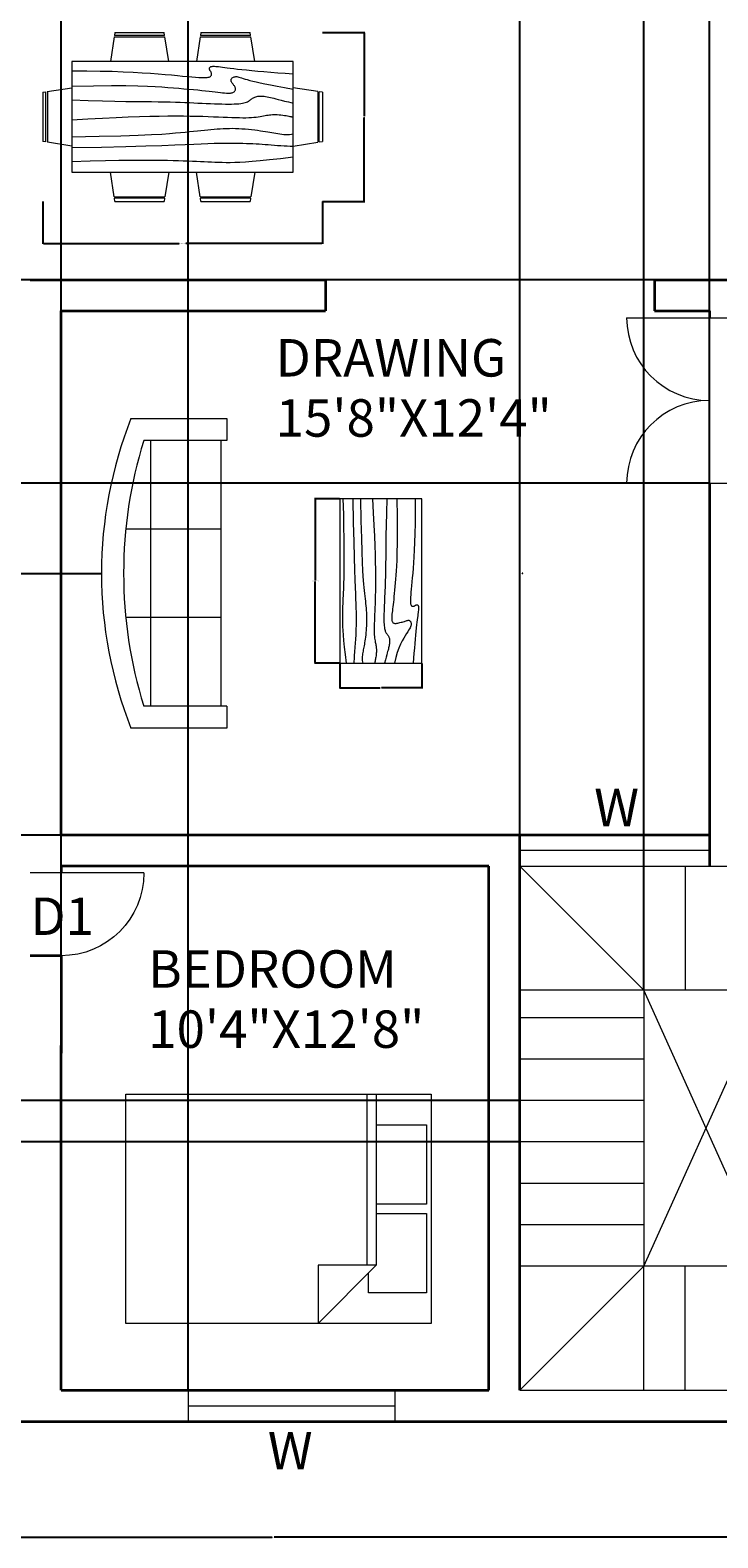
# Model space of a CAD drawing. Units: feet. Extents: x 1681 to 2398, y 1737 to 2411.
# Tile 2 of 4: x 1957 to 2156, y 1737 to 2174. Entities that reach past the tile are written whole.
import ezdxf

# ---------------------------------------------------------------- set-up
doc = ezdxf.new("R2010")
doc.units = ezdxf.units.FT
for name, color, linetype, lineweight in [('A-ANNO-DIMS', 2, 'Continuous', 18), ('A-ANNO-TEXT', 7, 'Continuous', 18), ('A-AREA-IDEN', 7, 'Continuous', 18), ('A-DOOR', 3, 'Continuous', 18), ('A-FLOR', 7, 'Continuous', 25), ('A-FLOR-STRS', 7, 'Continuous', 18), ('A-FURN', 8, 'Continuous', 13), ('A-GLAZ', 4, 'Continuous', 18), ('A-WALL', 7, 'Continuous', 35)]:
    doc.layers.add(name, color=color, linetype=linetype, lineweight=lineweight)
doc.styles.get("Standard").update_dxf_attribs({"font": 'arial.ttf'})
doc.dimstyles.get("Standard").update_dxf_attribs({"dimtxt": 0.18, "dimasz": 0.18, "dimexe": 0.18, "dimexo": 0.0625, "dimgap": 0.09, "dimtad": 0, "dimtih": 1, "dimtoh": 1, "dimdec": 4, "dimzin": 0, "dimdsep": 46, "dimtxsty": 'Standard', "dimcen": 0.09, "dimadec": 0, "dimazin": 0, "dimtfac": 1, "dimtdec": 4, "dimtofl": 0, "dimtmove": 0, "dimatfit": 3, "dimfxl": 1, "dimtolj": 1, "dimtzin": 0, "dimarcsym": 0})

# ---------------------------------------------------------------- blocks, each defined once
blk = doc.blocks.new('Dining Set - 36 x 72 in.')
for p, q in [((-22.2343, 26.00059), (-23.4847, 17.99762)), ((-22.2304, 26), (-5.7608, 26)), ((-22, 27.5), (-22.1562, 26.50042)), ((-5.8416, 26.5), (-22.1534, 26.5)), ((-22, 27.5), (-6, 27.5)), ((-5.8437, 26.49966), (-6, 27.5)), ((-4.5152, 17.99762), (-5.7655, 25.99926)), ((5.7657, 26.00059), (4.5153, 17.99762)), ((5.7696, 26), (22.2392, 26)), ((6, 27.5), (5.8438, 26.50042)), ((22.1584, 26.5), (5.8466, 26.5)), ((6, 27.5), (22, 27.5)), ((22.1563, 26.49966), (22, 27.5)), ((23.4848, 17.99762), (22.2345, 25.99926)), ((36, 18), (-36, 18)), ((-36, 18), (-36, -18)), ((36, -18), (36, 18)), ((-45.5, 8), (-44.5004, 8.15617)), ((-45.5, 8), (-45.5, -8)), ((-44.5, -8.15843), (-44.5, 8.15338)), ((-44.0006, 8.23428), (-35.9976, 9.48474)), ((-44, 8.23041), (-44, -8.23915)), ((44.0006, 8.23428), (35.9976, 9.48474)), ((44, 8.23041), (44, -8.23915)), ((44.5, -8.15843), (44.5, 8.15338)), ((45.5, 8), (44.5005, 8.15617)), ((45.5, 8), (45.5, -8)), ((-44.4997, -8.15631), (-45.5, -8)), ((-35.9976, -9.48476), (-43.9993, -8.2345)), ((35.9976, -9.48476), (43.9993, -8.2345)), ((44.4997, -8.15631), (45.5, -8)), ((-36, -18), (36, -18)), ((-22.2343, -26.0006), (-23.4847, -17.99762)), ((-4.5152, -17.99762), (-5.7655, -25.99928)), ((5.7657, -26.0006), (4.5153, -17.99762)), ((23.4848, -17.99762), (22.2345, -25.99928)), ((-22.2304, -26), (-5.7608, -26)), ((-22, -27.5), (-22.1562, -26.50044)), ((-5.8416, -26.5), (-22.1534, -26.5)), ((-22, -27.5), (-6, -27.5)), ((-5.8437, -26.49967), (-6, -27.5)), ((5.7696, -26), (22.2392, -26)), ((6, -27.5), (5.8438, -26.50044)), ((22.1584, -26.5), (5.8466, -26.5)), ((6, -27.5), (22, -27.5)), ((22.1563, -26.49967), (22, -27.5))]:
    blk.add_line(p, q)
for points in [[(-36, 15), (-31.1772, 14.97754), (-26.8079, 14.91406), (-22.8538, 14.81543), (-19.276, 14.6875), (-16.0362, 14.53613), (-13.0957, 14.36718), (-10.4159, 14.18652), (-7.9583, 14), (-5.6904, 13.81315), (-3.6035, 13.63021), (-1.6954, 13.45508), (0.0365, 13.29166), (1.5945, 13.14388), (2.9811, 13.01562), (4.1988, 12.9108), (5.25, 12.83333), (6.1393, 12.78613), (6.8802, 12.76823), (7.4883, 12.77767), (7.9792, 12.8125), (8.3685, 12.87077), (8.6719, 12.95052), (8.9049, 13.0498), (9.0833, 13.16666), (9.2205, 13.29899), (9.3216, 13.44401), (9.3895, 13.59879), (9.4271, 13.76041), (9.4373, 13.92594), (9.4232, 14.09245), (9.3875, 14.257), (9.3333, 14.41666), (9.2638, 14.56917), (9.1836, 14.71484), (9.0975, 14.85465), (9.0104, 14.98958), (8.9272, 15.1206), (8.8529, 15.2487), (8.7922, 15.37483), (8.75, 15.5), (8.7305, 15.62467), (8.7344, 15.74739), (8.7617, 15.86621), (8.8125, 15.97916), (8.8867, 16.08431), (8.9844, 16.17968), (9.1055, 16.26334), (9.25, 16.33333), (9.4189, 16.38802), (9.6172, 16.42708), (9.8506, 16.45052), (10.125, 16.45833), (10.4463, 16.45052), (10.8203, 16.42708), (11.2529, 16.38802), (11.75, 16.33333), (12.3184, 16.26318), (12.9694, 16.17838), (13.7151, 16.07991), (14.5677, 15.96875), (15.5395, 15.84586), (16.6426, 15.71224), (17.8893, 15.56884), (19.2917, 15.41666), (20.859, 15.25667), (22.5879, 15.08984), (24.4721, 14.91715), (26.5052, 14.73958), (28.6809, 14.5581), (30.9929, 14.3737), (33.4347, 14.18733), (36, 14)], [(-36, 10), (-28.9766, 10.14274), (-23.1725, 10.20442), (-18.4241, 10.19775), (-14.5677, 10.13541), (-11.4399, 10.03011), (-8.877, 9.89453), (-6.7154, 9.74137), (-4.7917, 9.58333), (-2.9698, 9.43082), (-1.2246, 9.28515), (0.4415, 9.14534), (2.026, 9.01041), (3.5266, 8.87939), (4.9408, 8.7513), (6.266, 8.62516), (7.5, 8.5), (8.6411, 8.37549), (9.6914, 8.2539), (10.6538, 8.13818), (11.5312, 8.03125), (12.3267, 7.93603), (13.043, 7.85547), (13.6831, 7.79248), (14.25, 7.75), (14.7471, 7.7303), (15.1797, 7.73307), (15.5537, 7.75732), (15.875, 7.80208), (16.1494, 7.86637), (16.3828, 7.94922), (16.5811, 8.04964), (16.75, 8.16666), (16.8944, 8.29915), (17.0143, 8.44531), (17.1089, 8.60319), (17.1771, 8.77083), (17.218, 8.94629), (17.2305, 9.1276), (17.2137, 9.31282), (17.1667, 9.5), (17.0895, 9.6875), (16.987, 9.875), (16.8649, 10.0625), (16.7292, 10.25), (16.5856, 10.4375), (16.4401, 10.625), (16.2985, 10.8125), (16.1667, 11), (16.05, 11.18733), (15.9518, 11.3737), (15.8752, 11.5581), (15.8229, 11.73958), (15.798, 11.91715), (15.8034, 12.08984), (15.842, 12.25667), (15.9167, 12.41666), (16.0295, 12.56836), (16.1784, 12.70833), (16.3605, 12.83268), (16.5729, 12.9375), (16.8127, 13.01888), (17.0768, 13.07291), (17.3625, 13.0957), (17.6667, 13.08333), (17.9894, 13.03312), (18.3418, 12.94726), (18.7382, 12.82918), (19.1927, 12.68229), (19.7195, 12.51001), (20.3327, 12.31575), (21.0465, 12.10294), (21.875, 11.875), (22.8357, 11.63354), (23.959, 11.37304), (25.2786, 11.08618), (26.8282, 10.76562), (28.6414, 10.40405), (30.752, 9.99414), (33.1936, 9.52856), (36, 9)], [(-36, 5.5), (-30.7157, 5.3348), (-26.069, 5.20963), (-21.9946, 5.11767), (-18.4271, 5.05208), (-15.3009, 5.00602), (-12.5508, 4.97265), (-10.1112, 4.94515), (-7.9167, 4.91666), (-5.909, 4.88167), (-4.0586, 4.83984), (-2.3429, 4.79215), (-0.7396, 4.73958), (0.7739, 4.6831), (2.22, 4.6237), (3.6213, 4.56233), (5, 4.5), (6.373, 4.43782), (7.7344, 4.3776), (9.0723, 4.32129), (10.375, 4.27083), (11.6309, 4.22819), (12.8281, 4.19531), (13.9551, 4.17415), (15, 4.16666), (15.954, 4.17448), (16.819, 4.19791), (17.6001, 4.23698), (18.3021, 4.29166), (18.9299, 4.36198), (19.4883, 4.44791), (19.9823, 4.54948), (20.4167, 4.66666), (20.7969, 4.79899), (21.1302, 4.94401), (21.4245, 5.09879), (21.6875, 5.26041), (21.9271, 5.42594), (22.1511, 5.59245), (22.3672, 5.757), (22.5834, 5.91666), (22.8065, 6.06868), (23.0404, 6.21093), (23.2879, 6.34147), (23.5521, 6.45833), (23.8358, 6.55957), (24.142, 6.64323), (24.4735, 6.70735), (24.8334, 6.75), (25.2235, 6.76969), (25.642, 6.76692), (26.0858, 6.74267), (26.5521, 6.69791), (27.0379, 6.63362), (27.5404, 6.55078), (28.0565, 6.45036), (28.5834, 6.33333), (29.1242, 6.19987), (29.7071, 6.04687), (30.3661, 5.87044), (31.1354, 5.66666), (32.0493, 5.43164), (33.142, 5.16146), (34.4475, 4.85221), (36, 4.5)], [(-36, -1), (-30.7915, -0.6591), (-26.0195, -0.38216), (-21.6519, -0.16284), (-17.6563, 0.00521), (-14.0005, 0.12833), (-10.6523, 0.21289), (-7.5796, 0.26522), (-4.75, 0.29166), (-2.134, 0.29793), (0.2878, 0.28711), (2.5317, 0.26163), (4.6146, 0.22396), (6.5529, 0.17651), (8.3633, 0.12174), (10.0623, 0.06209), (11.6667, 0), (13.1899, -0.06201), (14.6341, -0.1211), (15.9982, -0.17432), (17.2813, -0.21875), (18.4823, -0.25147), (19.6003, -0.26953), (20.6343, -0.27002), (21.5834, -0.25), (22.4481, -0.20768), (23.2357, -0.14584), (23.9549, -0.06836), (24.6146, 0.02083), (25.2235, 0.11784), (25.7904, 0.21875), (26.3241, 0.31966), (26.8334, 0.41666), (27.3265, 0.50618), (27.8099, 0.58593), (28.2894, 0.65397), (28.7709, 0.70833), (29.2601, 0.74707), (29.763, 0.76823), (30.2855, 0.76985), (30.8334, 0.75), (31.4088, 0.70784), (31.9994, 0.64713), (32.589, 0.57275), (33.1615, 0.48958), (33.7008, 0.4025), (34.1908, 0.3164), (34.6153, 0.23616), (34.9584, 0.16666), (35.2099, 0.11165), (35.3848, 0.07031), (35.504, 0.04069), (35.5886, 0.02083), (35.6594, 0.00879), (35.7377, 0.0026), (35.8442, 0.00032), (36, 0)], [(-36, -6.5), (-27.1843, -6.31267), (-20.084, -6.1263), (-14.469, -5.9419), (-10.1094, -5.76042), (-6.7752, -5.58285), (-4.2363, -5.41016), (-2.2629, -5.24333), (-0.625, -5.08334), (0.8708, -4.93099), (2.2715, -4.78646), (3.5872, -4.64974), (4.8281, -4.52084), (6.0046, -4.39974), (7.127, -4.28646), (8.2053, -4.18099), (9.25, -4.08334), (10.2705, -3.99382), (11.2734, -3.91407), (12.2647, -3.84603), (13.25, -3.79167), (14.2354, -3.75293), (15.2266, -3.73177), (16.2295, -3.73015), (17.25, -3.75), (18.2912, -3.79248), (19.3451, -3.85547), (20.4009, -3.93604), (21.4479, -4.03125), (22.4754, -4.13819), (23.4727, -4.25391), (24.4289, -4.37549), (25.3334, -4.5), (26.1785, -4.62492), (26.9694, -4.74935), (27.7145, -4.87281), (28.4219, -4.99479), (29.1, -5.11483), (29.7572, -5.23242), (30.4016, -5.34709), (31.0417, -5.45834), (31.6837, -5.56437), (32.3262, -5.65821), (32.9658, -5.73153), (33.599, -5.77604), (34.2224, -5.78345), (34.8327, -5.74545), (35.4264, -5.65373), (36, -5.5)], [(-36, -10), (-26.4022, -9.81299), (-18.4675, -9.62891), (-11.9839, -9.45069), (-6.7396, -9.28125), (-2.5226, -9.12354), (0.8789, -8.98047), (3.6769, -8.85498), (6.0833, -8.75), (8.2767, -8.66765), (10.3021, -8.60677), (12.1712, -8.56543), (13.8958, -8.54167), (15.4876, -8.53353), (16.9583, -8.53907), (18.3197, -8.55632), (19.5834, -8.58334), (20.7616, -8.61841), (21.8685, -8.66081), (22.9188, -8.71004), (23.9271, -8.76563), (24.9081, -8.82707), (25.8763, -8.89388), (26.8465, -8.96558), (27.8334, -9.04167), (28.8474, -9.12118), (29.8828, -9.20117), (30.93, -9.27824), (31.9792, -9.34896), (33.0205, -9.40991), (34.0443, -9.45768), (35.0407, -9.48885), (36, -9.5)], [(-36, -14.5), (-30.0881, -14.33513), (-25.0332, -14.21224), (-20.7312, -14.12647), (-17.0781, -14.07292), (-13.97, -14.04671), (-11.3027, -14.04297), (-8.9724, -14.05681), (-6.875, -14.08334), (-4.9224, -14.11833), (-3.0905, -14.16016), (-1.3709, -14.20785), (0.2448, -14.26042), (1.7647, -14.3169), (3.1973, -14.3763), (4.5507, -14.43767), (5.8333, -14.5), (7.0554, -14.5621), (8.235, -14.62175), (9.3922, -14.67652), (10.5469, -14.72396), (11.7192, -14.76164), (12.929, -14.78711), (14.1965, -14.79794), (15.5417, -14.79167), (16.9933, -14.76424), (18.6152, -14.70508), (20.4804, -14.60197), (22.6615, -14.44271), (25.2312, -14.21509), (28.2624, -13.9069), (31.8277, -13.50594), (36, -13)]]:
    blk.add_lwpolyline(points)
blk = doc.blocks.new('Bed - Queen')
for p, q in [((0, -80.00003), (0, 0)), ((0, 0), (59.99999, 0)), ((59.99999, 0), (59.99999, -80.00003)), ((7.99999, -1.2), (28.79998, -1.2)), ((7.99999, -14.4), (7.99999, -1.2)), ((28.79998, -1.2), (28.79998, -14.4)), ((31.19999, -1.2), (51.99999, -1.2)), ((31.19999, -14.4), (31.19999, -1.2)), ((51.99999, -1.2), (51.99999, -16.4)), ((0, -14.4), (44.8, -14.4)), ((59.99999, -29.6), (44.8, -14.4)), ((44.8, -14.4), (44.8, -29.6)), ((44.8, -16.8), (0, -16.8)), ((51.99999, -16.4), (46.79936, -16.4)), ((44.8, -29.6), (59.99999, -29.6)), ((59.99999, -80.00003), (0, -80.00003))]:
    blk.add_line(p, q)
blk = doc.blocks.new('Sofa - Roundback 7 ft.')
for p, q in [((-12.00002, -32.4421), (-12.00003, -6.5971)), ((11.99997, -32.4421), (11.99998, -6.5971)), ((-36.000027, -34), (-36.000027, -11.4696)), ((35.99998, -34), (35.99998, -11.4696)), ((-35.999844, -13.3819), (35.9998, -13.3819)), ((-36.000027, -32.4421), (35.99998, -32.4421))]:
    blk.add_line(p, q)
for points in [[(-36.000027, -34), (-42.000027, -34), (-42.000027, -8)], [(41.99998, -8), (41.99998, -34), (35.99998, -34)]]:
    blk.add_lwpolyline(points)
for centre, radius, start, end in [((0, -114.25), 114.25, 68.43141, 111.5686), ((-0.00001, -127.1968), 121.1968, 72.72033, 107.2797)]:
    blk.add_arc(centre, radius, start, end)
blk = doc.blocks.new('Table - Rectangular Woodgrain 60 x 30 in.')
for p, q in [((0, 0), (0, -30)), ((60, 0), (0, 0)), ((60, -30), (60, 0)), ((0, -30), (60, -30))]:
    blk.add_line(p, q)
for points in [[(0, -2.4), (4.8155, -2.418), (9.0302, -2.4688), (12.709, -2.5477), (15.9167, -2.65), (18.7181, -2.7711), (21.1781, -2.9063), (23.3616, -3.0508), (25.3333, -3.2), (27.1477, -3.3495), (28.8172, -3.4958), (30.3437, -3.636), (31.7291, -3.7667), (32.9756, -3.8849), (34.0849, -3.9875), (35.059, -4.0714), (35.9, -4.1334), (36.6114, -4.1711), (37.2041, -4.1854), (37.6906, -4.1779), (38.0833, -4.15), (38.3948, -4.1034), (38.6375, -4.0396), (38.8239, -3.9602), (38.9666, -3.8667), (39.0764, -3.7608), (39.1573, -3.6448), (39.2116, -3.521), (39.2416, -3.3917), (39.2498, -3.2593), (39.2385, -3.1261), (39.21, -2.9944), (39.1666, -2.8667), (39.111, -2.7447), (39.0468, -2.6281), (38.978, -2.5163), (38.9083, -2.4083), (38.8418, -2.3035), (38.7823, -2.201), (38.7337, -2.1001), (38.7, -2), (38.6844, -1.9003), (38.6875, -1.8021), (38.7094, -1.707), (38.75, -1.6167), (38.8094, -1.5326), (38.8875, -1.4563), (38.9844, -1.3893), (39.1, -1.3333), (39.2351, -1.2896), (39.3937, -1.2583), (39.5804, -1.2396), (39.8, -1.2333), (40.057, -1.2396), (40.3562, -1.2583), (40.7023, -1.2896), (41.1, -1.3333), (41.5547, -1.3895), (42.0755, -1.4573), (42.6721, -1.5361), (43.3542, -1.625), (44.1316, -1.7233), (45.014, -1.8302), (46.0114, -1.9449), (47.1333, -2.0667), (48.3862, -2.1947), (49.7625, -2.3281), (51.2513, -2.4663), (52.8416, -2.6083), (54.5226, -2.7535), (56.2833, -2.9011), (58.1127, -3.0501), (60, -3.2)], [(0, -9.2), (6.5759, -9.0858), (11.9385, -9.0365), (16.2527, -9.0418), (19.6833, -9.0917), (22.3952, -9.1759), (24.5531, -9.2844), (26.322, -9.4069), (27.8666, -9.5333), (29.3241, -9.6553), (30.7203, -9.7719), (32.0532, -9.8837), (33.3208, -9.9917), (34.5213, -10.0965), (35.6526, -10.199), (36.7128, -10.2999), (37.7, -10.4), (38.6129, -10.4996), (39.4531, -10.5969), (40.223, -10.6895), (40.925, -10.775), (41.5613, -10.8512), (42.1344, -10.9156), (42.6465, -10.966), (43.1, -11), (43.4976, -11.0158), (43.8437, -11.0136), (44.143, -10.9942), (44.4, -10.9583), (44.6195, -10.9069), (44.8062, -10.8406), (44.9648, -10.7603), (45.1, -10.6667), (45.2155, -10.5598), (45.3114, -10.4365), (45.3871, -10.2929), (45.4416, -10.125), (45.4743, -9.929), (45.4844, -9.7011), (45.4709, -9.4371), (45.4333, -9.1333), (45.3716, -8.7883), (45.2896, -8.4104), (45.1919, -8.0107), (45.0833, -7.6), (44.9685, -7.1893), (44.8521, -6.7896), (44.7388, -6.4117), (44.6333, -6.0667), (44.54, -5.7628), (44.4614, -5.4979), (44.4001, -5.2675), (44.3583, -5.0667), (44.3384, -4.8909), (44.3427, -4.7354), (44.3736, -4.5956), (44.4333, -4.4667), (44.5236, -4.3453), (44.6427, -4.2333), (44.7884, -4.1339), (44.9583, -4.05), (45.1501, -3.9849), (45.3614, -3.9417), (45.59, -3.9234), (45.8333, -3.9333), (46.0915, -3.9749), (46.3734, -4.0531), (46.6906, -4.1736), (47.0542, -4.3417), (47.4756, -4.5629), (47.9661, -4.8427), (48.5372, -5.1866), (49.2, -5.6), (49.9676, -6.0844), (50.8594, -6.625), (51.8965, -7.2031), (53.1, -7.8), (54.491, -8.3969), (56.0906, -8.975), (57.9199, -9.5156), (60, -10)], [(0, -12.8), (5.1847, -12.9322), (9.6213, -13.0323), (13.3963, -13.1059), (16.5958, -13.1583), (19.3063, -13.1952), (21.614, -13.2219), (23.6054, -13.2439), (25.3666, -13.2667), (26.9728, -13.2947), (28.4531, -13.3281), (29.8256, -13.3663), (31.1083, -13.4083), (32.3191, -13.4535), (33.476, -13.501), (34.597, -13.5501), (35.7, -13.6), (36.7984, -13.6497), (37.8875, -13.6979), (38.9578, -13.743), (40, -13.7833), (41.0047, -13.8174), (41.9625, -13.8438), (42.864, -13.8607), (43.7, -13.8667), (44.4631, -13.8604), (45.1552, -13.8417), (45.7801, -13.8104), (46.3416, -13.7667), (46.8439, -13.7104), (47.2906, -13.6417), (47.6858, -13.5604), (48.0333, -13.4667), (48.3375, -13.3608), (48.6042, -13.2448), (48.8396, -13.121), (49.05, -12.9917), (49.2417, -12.8593), (49.4208, -12.7261), (49.5937, -12.5944), (49.7667, -12.4667), (49.9452, -12.3451), (50.1323, -12.2313), (50.3303, -12.1268), (50.5416, -12.0333), (50.7686, -11.9524), (51.0135, -11.8854), (51.2788, -11.8341), (51.5666, -11.8), (51.8785, -11.7843), (52.2116, -11.7865), (52.562, -11.8059), (52.926, -11.8417), (53.2998, -11.8931), (53.6795, -11.9594), (54.0614, -12.0397), (54.4416, -12.1333), (54.8223, -12.2401), (55.2293, -12.3625), (55.6942, -12.5037), (56.2489, -12.6667), (56.9251, -12.8547), (57.7545, -13.0708), (58.7689, -13.3182), (60, -13.6)], [(0, -18), (5.124, -17.7273), (9.6609, -17.5057), (13.6705, -17.3303), (17.2125, -17.1958), (20.3467, -17.0973), (23.1328, -17.0297), (25.6307, -16.9878), (27.9, -16.9667), (29.9928, -16.9617), (31.9302, -16.9703), (33.7254, -16.9907), (35.3917, -17.0208), (36.9423, -17.0588), (38.3906, -17.1026), (39.7499, -17.1503), (41.0333, -17.2), (42.2519, -17.2496), (43.4073, -17.2969), (44.4986, -17.3395), (45.525, -17.375), (46.4858, -17.4012), (47.3802, -17.4156), (48.2074, -17.416), (48.9667, -17.4), (49.6583, -17.3662), (50.2872, -17.3167), (50.8595, -17.2547), (51.3812, -17.1833), (51.8584, -17.1057), (52.2971, -17.025), (52.7034, -16.9443), (53.0833, -16.8667), (53.443, -16.7951), (53.789, -16.7313), (54.128, -16.6768), (54.4666, -16.6334), (54.8115, -16.6024), (55.1693, -16.5854), (55.5465, -16.5841), (55.95, -16.6), (56.3828, -16.6337), (56.8346, -16.6823), (57.2915, -16.7418), (57.7396, -16.8084), (58.165, -16.878), (58.5539, -16.9469), (58.8924, -17.0111), (59.1666, -17.0667), (59.3679, -17.1107), (59.5078, -17.1438), (59.6032, -17.1675), (59.6708, -17.1833), (59.7275, -17.193), (59.7901, -17.1979), (59.8753, -17.1998), (60, -17.2)], [(0, -22.4), (8.0098, -22.2501), (14.4094, -22.1011), (19.4168, -21.9535), (23.25, -21.8083), (26.1269, -21.6663), (28.2656, -21.5281), (29.884, -21.3947), (31.2, -21.2667), (32.3967, -21.1448), (33.5172, -21.0292), (34.5697, -20.9198), (35.5625, -20.8167), (36.5037, -20.7198), (37.4015, -20.6292), (38.2642, -20.5448), (39.1, -20.4667), (39.9164, -20.3951), (40.7187, -20.3313), (41.5117, -20.2768), (42.3, -20.2333), (43.0883, -20.2024), (43.8812, -20.1854), (44.6836, -20.1841), (45.5, -20.2), (46.3328, -20.234), (47.1747, -20.2844), (48.0163, -20.3488), (48.8479, -20.425), (49.66, -20.5106), (50.4429, -20.6031), (51.1872, -20.7004), (51.8833, -20.8), (52.5246, -20.8999), (53.1166, -20.9995), (53.6681, -21.0983), (54.1875, -21.1958), (54.6834, -21.2919), (55.1646, -21.3859), (55.6394, -21.4777), (56.1167, -21.5667), (56.6028, -21.6515), (57.0961, -21.7266), (57.5929, -21.7852), (58.0896, -21.8208), (58.5823, -21.8268), (59.0674, -21.7964), (59.5412, -21.723), (60, -21.6)], [(0, -25.2), (8.6355, -25.0504), (15.7026, -24.9031), (21.4049, -24.7606), (25.9458, -24.625), (29.529, -24.4988), (32.3578, -24.3844), (34.6359, -24.284), (36.5667, -24.2), (38.3213, -24.1341), (39.9417, -24.0854), (41.437, -24.0523), (42.8167, -24.0333), (44.0901, -24.0268), (45.2667, -24.0313), (46.3557, -24.0451), (47.3667, -24.0667), (48.309, -24.0947), (49.1928, -24.1287), (50.0284, -24.168), (50.826, -24.2125), (51.5959, -24.2617), (52.3483, -24.3151), (53.0935, -24.3725), (53.8417, -24.4334), (54.6009, -24.497), (55.3699, -24.561), (56.1454, -24.6226), (56.9239, -24.6792), (57.7021, -24.7279), (58.4764, -24.7662), (59.2435, -24.7911), (60, -24.8)], [(0, -28.8), (5.6867, -28.6681), (10.45, -28.5698), (14.407, -28.5012), (17.675, -28.4584), (20.3711, -28.4374), (22.6125, -28.4344), (24.5164, -28.4455), (26.2, -28.4667), (27.762, -28.4947), (29.2276, -28.5281), (30.6033, -28.5663), (31.8958, -28.6084), (33.1118, -28.6535), (34.2578, -28.7011), (35.3405, -28.7501), (36.3666, -28.8), (37.3443, -28.8497), (38.288, -28.8974), (39.2137, -28.9412), (40.1375, -28.9792), (41.0753, -29.0093), (42.0432, -29.0297), (43.0572, -29.0384), (44.1333, -29.0333), (45.2936, -29.0114), (46.5843, -28.9641), (48.0579, -28.8816), (49.7666, -28.7542), (51.7629, -28.5721), (54.0989, -28.3255), (56.8272, -28.0048), (60, -27.6)]]:
    blk.add_lwpolyline(points)
blk = doc.blocks.new('DOOR-SINGLE-SWING')
blk.add_line((33, 0), (0, 0))
blk.add_arc((9, 0), 24, 0, 90)
blk = doc.blocks.new('DOOR-DOUBLE-SWING')
for p, q in [((0, 48), (33, 48)), ((0, 0), (33, 0))]:
    blk.add_line(p, q)
for centre, start, end in [((24, 48), 180, 270), ((24, 0), 90, 180)]:
    blk.add_arc(centre, 24, start, end)
blk = doc.blocks.new('WINDOW-STANDARD')
for p, q in [((0, 9), (0, 0)), ((60, 9), (60, 0)), ((0, 4.5), (60, 4.5))]:
    blk.add_line(p, q)
blk = doc.blocks.new('*D28')
at = {"layer": 'A-ANNO-DIMS', "color": 0, "lineweight": -2, "transparency": 16777216}
for p, q in [((2046.46, 2038.55), (2039.19, 2038.55)), ((2039.37, 2038.37), (2039.37, 2014.89)), ((2039.37, 1991.05), (2039.37, 2014.52)), ((2046.46, 1990.87), (2039.19, 1990.87))]:
    blk.add_line(p, q, dxfattribs=at)
at = {"layer": 'A-ANNO-DIMS', "color": 0, "transparency": 16777216}
for points in [[(2039.34, 2038.37), (2039.4, 2038.37), (2039.37, 2038.55)], [(2039.34, 1991.05), (2039.4, 1991.05), (2039.37, 1990.87)]]:
    blk.add_solid(points, dxfattribs=at)
at = {"layer": 'Defpoints', "color": 0, "transparency": 16777216}
for p in [(2046.52, 2038.55), (2039.37, 1990.87), (2046.52, 1990.87)]:
    blk.add_point(p, dxfattribs=at)
at = {"layer": 'A-ANNO-DIMS', "color": 0, "transparency": 16777216, "insert": (2039.37, 2014.71), "char_height": 0.18, "attachment_point": 5}
blk.add_mtext('\\A1;COFFEE TABLE 48', dxfattribs=at)
blk = doc.blocks.new('*D29')
at = {"layer": 'A-ANNO-DIMS', "color": 0, "lineweight": -2, "transparency": 16777216}
for p, q in [((2046.52, 1990.81), (2046.52, 1983.54)), ((2070.36, 1990.81), (2070.36, 1983.54)), ((2046.7, 1983.72), (2058.22, 1983.72)), ((2070.18, 1983.72), (2058.66, 1983.72))]:
    blk.add_line(p, q, dxfattribs=at)
at = {"layer": 'A-ANNO-DIMS', "color": 0, "transparency": 16777216}
for points in [[(2046.7, 1983.75), (2046.7, 1983.69), (2046.52, 1983.72)], [(2070.18, 1983.75), (2070.18, 1983.69), (2070.36, 1983.72)]]:
    blk.add_solid(points, dxfattribs=at)
at = {"layer": 'Defpoints', "color": 0, "transparency": 16777216}
for p in [(2046.52, 1990.87), (2070.36, 1990.87), (2070.36, 1983.72)]:
    blk.add_point(p, dxfattribs=at)
at = {"layer": 'A-ANNO-DIMS', "color": 0, "transparency": 16777216, "insert": (2058.44, 1983.72), "char_height": 0.18, "attachment_point": 5}
blk.add_mtext('\\A1;24', dxfattribs=at)
blk = doc.blocks.new('*D36')
at = {"layer": 'A-ANNO-DIMS', "color": 0, "lineweight": -2, "transparency": 16777216}
for p, q in [((1960.39, 2124.7), (1960.39, 2112.42)), ((2041.49, 2124.7), (2041.49, 2112.42)), ((1960.57, 2112.6), (1999.99, 2112.6)), ((2041.31, 2112.6), (2001.89, 2112.6))]:
    blk.add_line(p, q, dxfattribs=at)
at = {"layer": 'A-ANNO-DIMS', "color": 0, "transparency": 16777216}
for points in [[(1960.57, 2112.63), (1960.57, 2112.57), (1960.39, 2112.6)], [(2041.31, 2112.63), (2041.31, 2112.57), (2041.49, 2112.6)]]:
    blk.add_solid(points, dxfattribs=at)
at = {"layer": 'Defpoints', "color": 0, "transparency": 16777216}
for p in [(1960.39, 2124.76), (2041.49, 2124.76), (2041.49, 2112.6)]:
    blk.add_point(p, dxfattribs=at)
at = {"layer": 'A-ANNO-DIMS', "color": 0, "transparency": 16777216, "insert": (2000.94, 2112.6), "char_height": 0.18, "attachment_point": 5}
blk.add_mtext('\\A1;DINING SET 81', dxfattribs=at)
blk = doc.blocks.new('*D37')
at = {"layer": 'A-ANNO-DIMS', "color": 0, "lineweight": -2, "transparency": 16777216}
for p, q in [((2041.55, 2173.78), (2053.84, 2173.78)), ((2053.66, 2173.6), (2053.66, 2149.46)), ((2053.66, 2124.94), (2053.66, 2149.09)), ((2041.55, 2124.76), (2053.84, 2124.76))]:
    blk.add_line(p, q, dxfattribs=at)
at = {"layer": 'A-ANNO-DIMS', "color": 0, "transparency": 16777216}
for points in [[(2053.63, 2173.6), (2053.69, 2173.6), (2053.66, 2173.78)], [(2053.63, 2124.94), (2053.69, 2124.94), (2053.66, 2124.76)]]:
    blk.add_solid(points, dxfattribs=at)
at = {"layer": 'Defpoints', "color": 0, "transparency": 16777216}
for p in [(2041.49, 2173.78), (2053.66, 2173.78), (2041.49, 2124.76)]:
    blk.add_point(p, dxfattribs=at)
at = {"layer": 'A-ANNO-DIMS', "color": 0, "transparency": 16777216, "insert": (2053.66, 2149.27), "char_height": 0.18, "attachment_point": 5}
blk.add_mtext('\\A1;49', dxfattribs=at)
blk = doc.blocks.new('*D40')
at = {"layer": 'A-ANNO-DIMS', "color": 0, "lineweight": -2, "transparency": 16777216}
for p, q in [((1714.74, 1770.99), (1714.74, 1737.27)), ((2339.74, 1770.99), (2339.74, 1737.27)), ((1714.92, 1737.45), (2026.95, 1737.45)), ((2339.56, 1737.45), (2027.53, 1737.45))]:
    blk.add_line(p, q, dxfattribs=at)
at = {"layer": 'A-ANNO-DIMS', "color": 0, "transparency": 16777216}
for points in [[(1714.92, 1737.48), (1714.92, 1737.42), (1714.74, 1737.45)], [(2339.56, 1737.48), (2339.56, 1737.42), (2339.74, 1737.45)]]:
    blk.add_solid(points, dxfattribs=at)
at = {"layer": 'Defpoints', "color": 0, "transparency": 16777216}
for p in [(1714.74, 1771.05), (2339.74, 1771.05), (2339.74, 1737.45)]:
    blk.add_point(p, dxfattribs=at)
at = {"layer": 'A-ANNO-DIMS', "color": 0, "transparency": 16777216, "insert": (2027.24, 1737.45), "char_height": 0.18, "attachment_point": 5}
blk.add_mtext('\\A1;625', dxfattribs=at)
blk = doc.blocks.new('*D50')
at = {"layer": 'A-ANNO-DIMS', "color": 0, "lineweight": -2, "transparency": 16777216}
for p, q in [((2330.68, 2232.39), (1680.96, 2232.39)), ((1681.14, 2232.21), (1681.14, 2167.4)), ((1681.14, 2102.23), (1681.14, 2167.04)), ((2330.68, 2102.05), (1680.96, 2102.05))]:
    blk.add_line(p, q, dxfattribs=at)
at = {"layer": 'A-ANNO-DIMS', "color": 0, "transparency": 16777216}
for points in [[(1681.11, 2232.21), (1681.17, 2232.21), (1681.14, 2232.39)], [(1681.11, 2102.23), (1681.17, 2102.23), (1681.14, 2102.05)]]:
    blk.add_solid(points, dxfattribs=at)
at = {"layer": 'Defpoints', "color": 0, "transparency": 16777216}
for p in [(1681.14, 2232.39), (2330.74, 2232.39), (2330.74, 2102.05)]:
    blk.add_point(p, dxfattribs=at)
at = {"layer": 'A-ANNO-DIMS', "color": 0, "transparency": 16777216, "insert": (1681.14, 2167.22), "char_height": 0.18, "attachment_point": 5}
blk.add_mtext('\\A1;130.34', dxfattribs=at)
blk = doc.blocks.new('*D52')
at = {"layer": 'A-ANNO-DIMS', "color": 0, "lineweight": -2, "transparency": 16777216}
for p, q in [((1965.74, 1780.11), (1965.74, 2410.83)), ((1965.92, 2410.65), (1983.77, 2410.65)), ((2002.37, 2410.65), (1984.52, 2410.65)), ((2002.55, 1780.11), (2002.55, 2410.83))]:
    blk.add_line(p, q, dxfattribs=at)
at = {"layer": 'A-ANNO-DIMS', "color": 0, "transparency": 16777216}
for points in [[(1965.92, 2410.68), (1965.92, 2410.62), (1965.74, 2410.65)], [(2002.37, 2410.68), (2002.37, 2410.62), (2002.55, 2410.65)]]:
    blk.add_solid(points, dxfattribs=at)
at = {"layer": 'Defpoints', "color": 0, "transparency": 16777216}
for p in [(2002.55, 2410.65), (1965.74, 1780.05), (2002.55, 1780.05)]:
    blk.add_point(p, dxfattribs=at)
at = {"layer": 'A-ANNO-DIMS', "color": 0, "transparency": 16777216, "insert": (1984.15, 2410.65), "char_height": 0.18, "attachment_point": 5}
blk.add_mtext('\\A1;36.81', dxfattribs=at)
blk = doc.blocks.new('*D53')
at = {"layer": 'A-ANNO-DIMS', "color": 0, "lineweight": -2, "transparency": 16777216}
for p, q in [((2098.74, 1816.11), (2098.74, 2410.83)), ((2098.92, 2410.65), (2146.52, 2410.65)), ((2194.56, 2410.65), (2146.96, 2410.65)), ((2194.74, 1816.11), (2194.74, 2410.83))]:
    blk.add_line(p, q, dxfattribs=at)
at = {"layer": 'A-ANNO-DIMS', "color": 0, "transparency": 16777216}
for points in [[(2098.92, 2410.68), (2098.92, 2410.62), (2098.74, 2410.65)], [(2194.56, 2410.68), (2194.56, 2410.62), (2194.74, 2410.65)]]:
    blk.add_solid(points, dxfattribs=at)
at = {"layer": 'Defpoints', "color": 0, "transparency": 16777216}
for p in [(2194.74, 2410.65), (2098.74, 1816.05), (2194.74, 1816.05)]:
    blk.add_point(p, dxfattribs=at)
at = {"layer": 'A-ANNO-DIMS', "color": 0, "transparency": 16777216, "insert": (2146.74, 2410.65), "char_height": 0.18, "attachment_point": 5}
blk.add_mtext('\\A1;96', dxfattribs=at)
blk = doc.blocks.new('*D55')
at = {"layer": 'A-ANNO-DIMS', "color": 0, "lineweight": -2, "transparency": 16777216}
for p, q in [((2098.74, 1896.11), (2098.74, 2410.83)), ((2098.92, 2410.65), (2116.52, 2410.65)), ((2134.56, 2410.65), (2116.96, 2410.65)), ((2134.74, 1896.11), (2134.74, 2410.83))]:
    blk.add_line(p, q, dxfattribs=at)
at = {"layer": 'A-ANNO-DIMS', "color": 0, "transparency": 16777216}
for points in [[(2098.92, 2410.68), (2098.92, 2410.62), (2098.74, 2410.65)], [(2134.56, 2410.68), (2134.56, 2410.62), (2134.74, 2410.65)]]:
    blk.add_solid(points, dxfattribs=at)
at = {"layer": 'Defpoints', "color": 0, "transparency": 16777216}
for p in [(2098.74, 2410.65), (2098.74, 1896.05), (2134.74, 1896.05)]:
    blk.add_point(p, dxfattribs=at)
at = {"layer": 'A-ANNO-DIMS', "color": 0, "transparency": 16777216, "insert": (2116.74, 2410.65), "char_height": 0.18, "attachment_point": 5}
blk.add_mtext('\\A1;36', dxfattribs=at)
blk = doc.blocks.new('*D57')
at = {"layer": 'A-ANNO-DIMS', "color": 0, "lineweight": -2, "transparency": 16777216}
for p, q in [((2153.68, 2043.05), (1680.96, 2043.05)), ((1681.14, 2042.87), (1681.14, 1992.23)), ((1681.14, 1941.23), (1681.14, 1991.87)), ((2153.68, 1941.05), (1680.96, 1941.05))]:
    blk.add_line(p, q, dxfattribs=at)
at = {"layer": 'A-ANNO-DIMS', "color": 0, "transparency": 16777216}
for points in [[(1681.11, 2042.87), (1681.17, 2042.87), (1681.14, 2043.05)], [(1681.11, 1941.23), (1681.17, 1941.23), (1681.14, 1941.05)]]:
    blk.add_solid(points, dxfattribs=at)
at = {"layer": 'Defpoints', "color": 0, "transparency": 16777216}
for p in [(1681.14, 2043.05), (2153.74, 2043.05), (2153.74, 1941.05)]:
    blk.add_point(p, dxfattribs=at)
at = {"layer": 'A-ANNO-DIMS', "color": 0, "transparency": 16777216, "insert": (1681.14, 1992.05), "char_height": 0.18, "attachment_point": 5}
blk.add_mtext('\\A1;102', dxfattribs=at)
blk = doc.blocks.new('*D59')
at = {"layer": 'A-ANNO-DIMS', "color": 0, "lineweight": -2, "transparency": 16777216}
for p, q in [((2098.74, 1941.11), (2098.74, 2410.83)), ((2098.92, 2410.65), (2126.02, 2410.65)), ((2153.56, 2410.65), (2126.46, 2410.65)), ((2153.74, 1941.11), (2153.74, 2410.83))]:
    blk.add_line(p, q, dxfattribs=at)
at = {"layer": 'A-ANNO-DIMS', "color": 0, "transparency": 16777216}
for points in [[(2098.92, 2410.68), (2098.92, 2410.62), (2098.74, 2410.65)], [(2153.56, 2410.68), (2153.56, 2410.62), (2153.74, 2410.65)]]:
    blk.add_solid(points, dxfattribs=at)
at = {"layer": 'Defpoints', "color": 0, "transparency": 16777216}
for p in [(2153.74, 2410.65), (2098.74, 1941.05), (2153.74, 1941.05)]:
    blk.add_point(p, dxfattribs=at)
at = {"layer": 'A-ANNO-DIMS', "color": 0, "transparency": 16777216, "insert": (2126.24, 2410.65), "char_height": 0.18, "attachment_point": 5}
blk.add_mtext('\\A1;55', dxfattribs=at)
blk = doc.blocks.new('*D62')
at = {"layer": 'A-ANNO-DIMS', "color": 0, "lineweight": -2, "transparency": 16777216}
for p, q in [((2098.68, 1864.05), (1680.96, 1864.05)), ((1681.14, 1863.87), (1681.14, 1858.23)), ((1681.14, 1852.23), (1681.14, 1857.87)), ((2098.68, 1852.05), (1680.96, 1852.05))]:
    blk.add_line(p, q, dxfattribs=at)
at = {"layer": 'A-ANNO-DIMS', "color": 0, "transparency": 16777216}
for points in [[(1681.11, 1863.87), (1681.17, 1863.87), (1681.14, 1864.05)], [(1681.11, 1852.23), (1681.17, 1852.23), (1681.14, 1852.05)]]:
    blk.add_solid(points, dxfattribs=at)
at = {"layer": 'Defpoints', "color": 0, "transparency": 16777216}
for p in [(1681.14, 1864.05), (2098.74, 1864.05), (2098.74, 1852.05)]:
    blk.add_point(p, dxfattribs=at)
at = {"layer": 'A-ANNO-DIMS', "color": 0, "transparency": 16777216, "insert": (1681.14, 1858.05), "char_height": 0.18, "attachment_point": 5}
blk.add_mtext('\\A1;12', dxfattribs=at)
blk = doc.blocks.new('*D65')
at = {"layer": 'A-ANNO-DIMS', "color": 0, "lineweight": -2, "transparency": 16777216}
for p, q in [((1904.14, 2016.92), (1977.25, 2016.92)), ((2099.48, 2016.93), (2099.66, 2016.93)), ((2099.57, 2016.84), (2099.57, 2017.02))]:
    blk.add_line(p, q, dxfattribs=at)
at = {"layer": 'A-ANNO-DIMS', "color": 0, "transparency": 16777216}
blk.add_solid([(1977.25, 2016.95), (1977.25, 2016.89), (1977.43, 2016.92)], dxfattribs=at)
at = {"layer": 'Defpoints', "color": 0, "transparency": 16777216}
for p in [(1977.43, 2016.92), (2099.57, 2016.93)]:
    blk.add_point(p, dxfattribs=at)
at = {"layer": 'A-ANNO-DIMS', "color": 0, "transparency": 16777216, "insert": (1903.4, 2016.92), "char_height": 0.18, "attachment_point": 5}
blk.add_mtext('\\A1;2X R122.14', dxfattribs=at)

msp = doc.modelspace()

# ---------------------------------------------------------------- linework, layer by layer
at = {"layer": 'A-FLOR'}
msp.add_line((1965.7402, 1771.0485), (2339.7402, 1771.0485), dxfattribs=at)
at = {"layer": 'A-FLOR-STRS'}
for p, q in [((2098.7402, 1932.0485), (2134.7402, 1932.0485)), ((2098.7402, 1932.0485), (2134.7402, 1896.0485)), ((2134.7402, 1932.0485), (2134.7402, 1816.0485)), ((2134.7402, 1932.0485), (2170.7402, 1932.0485)), ((2146.7402, 1932.0485), (2146.7402, 1896.0485)), ((2134.7402, 1896.0485), (2098.7402, 1896.0485)), ((2170.7402, 1896.0485), (2134.7402, 1896.0485)), ((2170.7402, 1816.0485), (2134.7402, 1896.0485)), ((2134.7402, 1816.0485), (2170.7402, 1896.0485)), ((2134.7402, 1888.0485), (2098.7402, 1888.0485)), ((2134.7402, 1876.0485), (2098.7402, 1876.0485)), ((2134.7402, 1864.0485), (2098.7402, 1864.0485)), ((2134.7402, 1852.0485), (2098.7402, 1852.0485)), ((2134.7402, 1840.0485), (2098.7402, 1840.0485)), ((2134.7402, 1828.0485), (2098.7402, 1828.0485)), ((2134.7402, 1816.0485), (2098.7402, 1816.0485)), ((2134.7402, 1816.0485), (2098.7402, 1780.0485)), ((2134.7402, 1780.0485), (2134.7402, 1816.0485)), ((2194.7402, 1816.0485), (2134.7402, 1816.0485)), ((2146.7402, 1780.0485), (2146.7402, 1816.0485)), ((2098.7402, 1780.0485), (2134.7402, 1780.0485)), ((2134.7402, 1780.0485), (2194.7402, 1780.0485))]:
    msp.add_line(p, q, dxfattribs=at)
at = {"layer": 'A-GLAZ'}
msp.add_line((2153.7402, 1936.5485), (2098.7402, 1936.5485), dxfattribs=at)
at = {"layer": 'A-WALL'}
for p, q in [((1956.7402, 2102.0485), (2042.3686, 2102.0485)), ((2042.3686, 2102.0485), (2042.3686, 2093.0485)), ((2137.7992, 2102.0485), (2137.7992, 2093.0485)), ((2137.7992, 2102.0485), (2227.2402, 2102.0485)), ((1965.7402, 1941.0485), (1965.7402, 2093.0485)), ((1965.7402, 2093.0485), (2042.3686, 2093.0485)), ((2137.7992, 2093.0485), (2153.7402, 2093.0485)), ((2153.7402, 2093.0485), (2153.7402, 2091.0485)), ((2153.7402, 2043.0485), (2153.7402, 1932.0485)), ((2153.7402, 1941.0485), (1965.7402, 1941.0485)), ((2098.7402, 1780.0485), (2098.7402, 1941.0485)), ((2089.7402, 1932.0485), (1965.7402, 1932.0485)), ((1965.7402, 1932.0485), (1965.7402, 1930.0485)), ((2089.7402, 1780.0485), (2089.7402, 1932.0485)), ((1965.7402, 1906.0485), (1956.7402, 1906.0485)), ((1965.7402, 1906.0485), (1965.7402, 1877.7891)), ((1965.7402, 1780.0485), (1965.7402, 1880.0485)), ((1965.7402, 1780.0485), (2089.7402, 1780.0485)), ((1714.7402, 1771.0485), (2194.7402, 1771.0485)), ((1880.7402, 1771.0485), (2194.7402, 1771.0485))]:
    msp.add_line(p, q, dxfattribs=at)

# ---------------------------------------------------------------- block references
at = {"layer": 'A-DOOR'}
msp.add_blockref('DOOR-DOUBLE-SWING', (2129.7402, 2043.0485), dxfattribs=at)
at = {"layer": 'A-DOOR', "extrusion": (0, 0, -1), "zscale": -1, "rotation": 180}
msp.add_blockref('DOOR-SINGLE-SWING', (-1956.7402, 1930.0485), dxfattribs=at)
at = {"layer": 'A-FURN', "xscale": 0.8912476229700672, "yscale": 0.8912476229700672, "zscale": 0.8912476229700672}
msp.add_blockref('Dining Set - 36 x 72 in.', (2000.9398, 2149.2743), dxfattribs=at)
at = {"layer": 'A-FURN'}
for name, p, xscale, yscale, zscale, rotation in [('Sofa - Roundback 7 ft.', (1977.4304, 2016.9252), 1.069080003544779, 1.069080003544779, 1.069080003544779, 89.99999999999999), ('Table - Rectangular Woodgrain 60 x 30 in.', (2070.3575, 2038.5455), 0.7946179109721978, 0.7946179109721978, 0.7946179109721978, 270), ('Bed - Queen', (2073.0498, 1865.8698), 1.106801235632363, 1.106801235632363, 1.106801235632363, 270)]:
    msp.add_blockref(name, p, dxfattribs=dict(at, xscale=xscale, yscale=yscale, zscale=zscale, rotation=rotation))
at = {"layer": 'A-GLAZ'}
msp.add_blockref('WINDOW-STANDARD', (2002.5532, 1771.0485), dxfattribs=at)

# ---------------------------------------------------------------- texts
at = {"layer": 'A-ANNO-TEXT'}
for s, height, p in [('W', 10.8568, (2120.3184, 1943.6079)), ('D1', 10.85679, (1956.8395, 1912.0729)), ('W', 10.8568, (2025.6672, 1757.1353))]:
    msp.add_text(s, height=height, dxfattribs=at).set_placement(p)
at = {"layer": 'A-AREA-IDEN'}
for s, height, p in [('DRAWING', 10.85679, (2027.9453, 2073.9855)), ('15\'8"X12\'4"', 10.856786, (2027.9453, 2056.545)), ('BEDROOM', 10.85679, (1990.9811, 1896.778)), ('10\'4"X12\'8"', 10.856786, (1990.9811, 1879.3375))]:
    msp.add_text(s, height=height, dxfattribs=at).set_placement(p)

# ---------------------------------------------------------------- dimensions: what is measured, and where the dimension line sits
at = {"layer": 'A-ANNO-DIMS'}
for base, p1, p2, override, picture, middle in [((2002.5532, 2410.6485), (1965.7402, 1780.0485), (2002.5532, 1780.0485), {"dimdec": 2, "dimlfac": 1, "dimrnd": 0, "dimzin": 0, "dimdsep": 46, "dimlunit": 2}, '*D52', (1984.1467, 2410.6485)), ((2194.7402, 2410.6485), (2098.7402, 1816.0485), (2194.7402, 1816.0485), {"dimdec": 0, "dimlfac": 1, "dimrnd": 0, "dimzin": 0, "dimdsep": 46, "dimlunit": 2}, '*D53', (2146.7402, 2410.6485)), ((2098.7402, 2410.6485), (2134.7402, 1896.0485), (2098.7402, 1896.0485), {"dimdec": 0, "dimlfac": 1, "dimrnd": 0, "dimzin": 0, "dimdsep": 46, "dimlunit": 2}, '*D55', (2116.7402, 2410.6485)), ((2153.7402, 2410.6485), (2098.7402, 1941.0485), (2153.7402, 1941.0485), {"dimdec": 0, "dimlfac": 1, "dimrnd": 0, "dimzin": 0, "dimdsep": 46, "dimlunit": 2}, '*D59', (2126.2402, 2410.6485)), ((2070.3575, 1983.7169), (2046.5189, 1990.8684), (2070.3575, 1990.8684), {"dimdec": 0, "dimlfac": 1, "dimrnd": 0, "dimzin": 0, "dimdsep": 46, "dimlunit": 2}, '*D29', (2058.4382, 1983.7169)), ((2339.7402, 1737.4485), (1714.7402, 1771.0485), (2339.7402, 1771.0485), {"dimdec": 0, "dimlfac": 1, "dimrnd": 0, "dimzin": 0, "dimdsep": 46, "dimlunit": 2}, '*D40', (2027.2402, 1737.4485))]:
    dim = msp.add_linear_dim(base=base, p1=p1, p2=p2, dimstyle='Standard', override=override, dxfattribs=at)
    dim.commit()
    dim.dimension.update_dxf_attribs({"geometry": picture, "text_midpoint": middle})
for base, p1, p2, override, picture, middle in [((1681.1402, 2232.3872), (2330.7402, 2102.0485), (2330.7402, 2232.3872), {"dimdec": 2, "dimlfac": 1, "dimrnd": 0, "dimzin": 0, "dimdsep": 46, "dimlunit": 2}, '*D50', (1681.1402, 2167.2178)), ((2053.6571, 2173.7836), (2041.4916, 2124.765), (2041.4916, 2173.7836), {"dimdec": 0, "dimlfac": 1, "dimrnd": 0, "dimzin": 0, "dimdsep": 46, "dimlunit": 2}, '*D37', (2053.6571, 2149.2743)), ((1681.1402, 2043.0485), (2153.7402, 1941.0485), (2153.7402, 2043.0485), {"dimdec": 0, "dimlfac": 1, "dimrnd": 0, "dimzin": 0, "dimdsep": 46, "dimlunit": 2}, '*D57', (1681.1402, 1992.0485)), ((1681.1402, 1864.0485), (2098.7402, 1852.0485), (2098.7402, 1864.0485), {"dimdec": 0, "dimlfac": 1, "dimrnd": 0, "dimzin": 0, "dimdsep": 46, "dimlunit": 2}, '*D62', (1681.1402, 1858.0485))]:
    dim = msp.add_linear_dim(base=base, p1=p1, p2=p2, angle=90, dimstyle='Standard', override=override, dxfattribs=at)
    dim.commit()
    dim.dimension.update_dxf_attribs({"geometry": picture, "text_midpoint": middle})
dim = msp.add_linear_dim(base=(2041.4916, 2112.5994), p1=(1960.3881, 2124.765), p2=(2041.4916, 2124.765), text='DINING SET <>', dimstyle='Standard', override={"dimdec": 0, "dimlfac": 1, "dimrnd": 0, "dimzin": 0, "dimdsep": 46, "dimlunit": 2}, dxfattribs=at)
dim.commit()
dim.dimension.update_dxf_attribs({"geometry": '*D36', "text_midpoint": (2000.9398, 2112.5994)})
dim = msp.add_linear_dim(base=(2039.3674, 1990.8684), p1=(2046.5189, 2038.5455), p2=(2046.5189, 1990.8684), angle=270, text='COFFEE TABLE <>', dimstyle='Standard', override={"dimdec": 0, "dimlfac": 1, "dimrnd": 0, "dimzin": 0, "dimdsep": 46, "dimlunit": 2}, dxfattribs=at)
dim.commit()
dim.dimension.update_dxf_attribs({"geometry": '*D28', "text_midpoint": (2039.3674, 2014.707)})
dim = msp.add_radius_dim(center=(2099.5728, 2016.9252), mpoint=(1977.4304, 2016.925), text='2X <>', dimstyle='Standard', override={"dimdec": 2, "dimlfac": 1, "dimrnd": 0, "dimzin": 0, "dimdsep": 46, "dimlunit": 2}, dxfattribs=at)
dim.commit()
dim.dimension.update_dxf_attribs({"geometry": '*D65', "text_midpoint": (1904.145, 2016.9249), "dimtype": 164})

doc.saveas('drawing.dxf')
